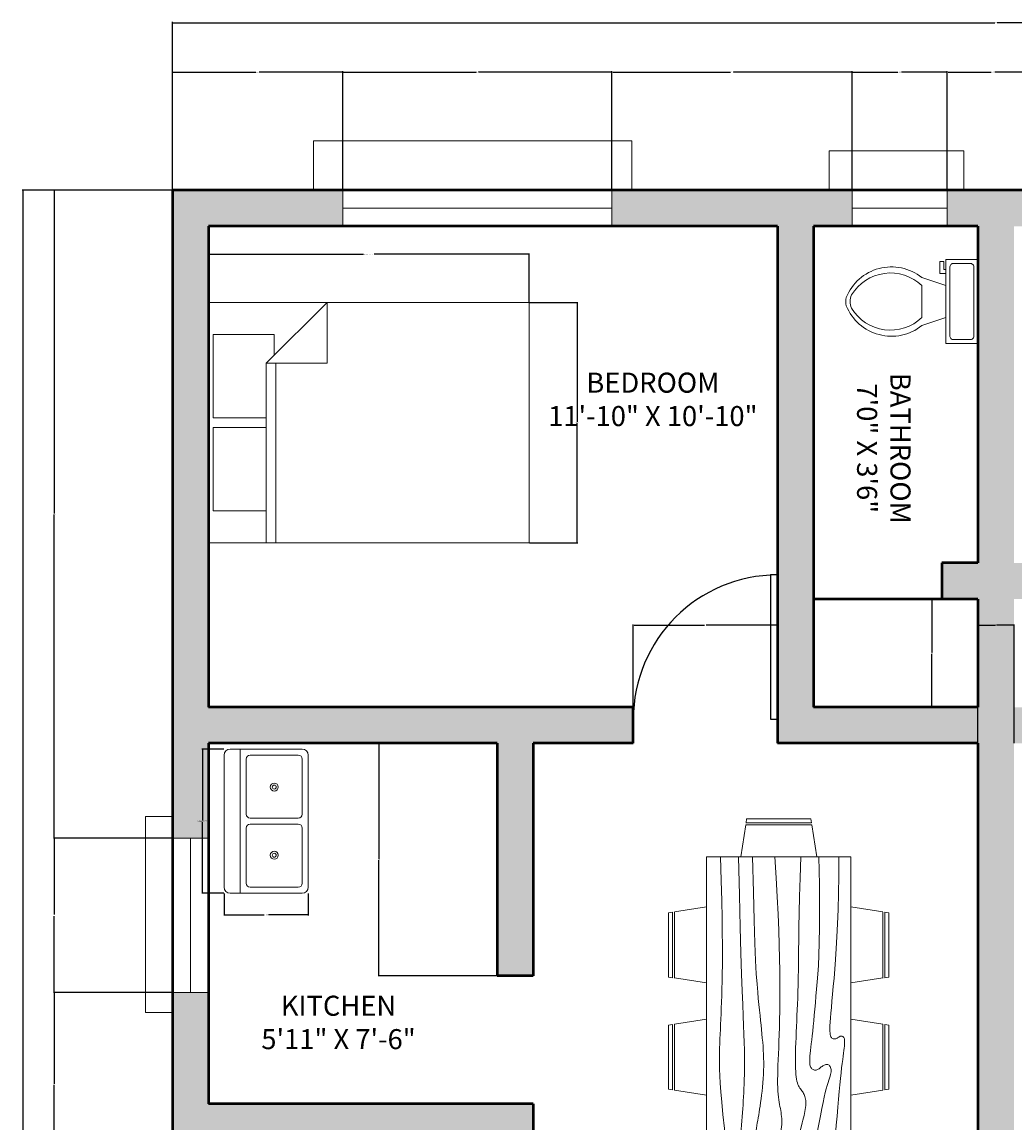
# Model space of a CAD drawing. Units: inches. Extents: x 2710 to 3197, y 524 to 1147.
# Tile 5 of 6: x 2710 to 2957, y 873 to 1147. Entities that reach past the tile are written whole.
import ezdxf

# ---------------------------------------------------------------- set-up
doc = ezdxf.new("R2010")
doc.units = ezdxf.units.IN
for name, color, linetype, lineweight in [('A-ANNO-DIMS', 2, 'Continuous', 18), ('A-AREA-IDEN', 7, 'Continuous', 25), ('A-DOOR', 3, 'Continuous', 25), ('A-FLOR-FIXT', 9, 'Continuous', 20), ('A-FURN', 8, 'Continuous', 18), ('A-GLAZ', 4, 'Continuous', 18), ('A-WALL', 7, 'Continuous', 50), ('A-WALL-PATT', 74, 'Continuous', 13)]:
    doc.layers.add(name, color=color, linetype=linetype, lineweight=lineweight)
doc.styles.get("Standard").update_dxf_attribs({"font": 'arial.ttf'})
doc.dimstyles.get("Standard").update_dxf_attribs({"dimtxt": 0.18, "dimasz": 0.18, "dimexe": 0.18, "dimexo": 0.0625, "dimgap": 0.09, "dimtad": 0, "dimtih": 1, "dimtoh": 1, "dimdec": 4, "dimzin": 0, "dimdsep": 46, "dimtxsty": 'Standard', "dimcen": 0.09, "dimadec": 0, "dimazin": 0, "dimtfac": 1, "dimtdec": 4, "dimtofl": 0, "dimtmove": 0, "dimatfit": 3, "dimfxl": 1, "dimtolj": 1, "dimtzin": 0, "dimarcsym": 0})

# ---------------------------------------------------------------- blocks, each defined once
blk = doc.blocks.new('*U5')
for p, q in [((0, 0), (0, -6)), ((-36, 0), (-36, -6))]:
    blk.add_line(p, q)
blk.add_lwpolyline([(0, 0), (0, 36), (-1.75, 36), (-1.75, 0)], close=True)
blk.add_arc((0, 0), 36, 90, 180)
blk = doc.blocks.new('Toilet - top')
for p, q in [((9.5, -6), (9.5, -2)), ((-8, -8.5), (-8, -8)), ((-7, -8), (-7, -9.5)), ((-4, -8), (-6, -14)), ((4, -8), (6, -14)), ((-10, -8.5), (-8, -8.5)), ((-10, -9.5), (-10, -8.5)), ((-7, -9.5), (-10, -9.5)), ((4, -14), (-4, -14))]:
    blk.add_line(p, q)
blk.add_lwpolyline([(10.5, -8), (10.5, 0), (-10.5, 0), (-10.5, -8)], close=True)
for points in [[(-9.5, -2), (-9.5, -6)], [(8.5, -1), (-8.5, -1)], [(-8.5, -7), (8.5, -7)]]:
    blk.add_lwpolyline(points)
for centre, radius, start, end in [((-8.62, -1.88), 0.884, 81.8699, 188.1301), ((8.62, -1.88), 0.884, 351.8699, 98.1301), ((-8.62, -6.12), 0.884, 171.8699, 278.1301), ((8.62, -6.12), 0.884, 261.8699, 8.1301), ((3.52, -21.58), 12.17, 141.4691, 247.9714), ((4.2, -21.82), 11.33, 136.3677, 238.9468), ((-3.52, -21.58), 12.17, 292.0284, 38.5307), ((-4.2, -21.82), 11.33, 301.053, 43.6321), ((0, -27.88), 4, 245.7318, 294.2682), ((0, -29), 4, 254.8605, 285.1395)]:
    blk.add_arc(centre, radius, start, end)
blk = doc.blocks.new('Bed - Queen')
for p, q in [((0, -80.00003), (0, 0)), ((0, 0), (59.99999, 0)), ((59.99999, 0), (59.99999, -80.00003)), ((7.99999, -1.2), (28.79998, -1.2)), ((7.99999, -14.4), (7.99999, -1.2)), ((28.79998, -1.2), (28.79998, -14.4)), ((31.19999, -1.2), (51.99999, -1.2)), ((31.19999, -14.4), (31.19999, -1.2)), ((51.99999, -1.2), (51.99999, -16.4)), ((0, -14.4), (44.8, -14.4)), ((59.99999, -29.6), (44.8, -14.4)), ((44.8, -14.4), (44.8, -29.6)), ((51.99999, -16.4), (46.79936, -16.4)), ((44.8, -16.8), (0, -16.8)), ((44.8, -29.6), (59.99999, -29.6)), ((59.99999, -80.00003), (0, -80.00003))]:
    blk.add_line(p, q)
blk = doc.blocks.new('Dining Set - 36 x 72 in.')
for p, q in [((-22, 27.5), (-22.1562, 26.50042)), ((-22, 27.5), (-6, 27.5)), ((-5.8437, 26.49966), (-6, 27.5)), ((6, 27.5), (5.8438, 26.50042)), ((6, 27.5), (22, 27.5)), ((22.1563, 26.49966), (22, 27.5)), ((-22.2343, 26.00059), (-23.4847, 17.99762)), ((-22.2304, 26), (-5.7608, 26)), ((-5.8416, 26.5), (-22.1534, 26.5)), ((-4.5152, 17.99762), (-5.7655, 25.99926)), ((5.7657, 26.00059), (4.5153, 17.99762)), ((5.7696, 26), (22.2392, 26)), ((22.1584, 26.5), (5.8466, 26.5)), ((23.4848, 17.99762), (22.2345, 25.99926)), ((36, 18), (-36, 18)), ((-36, 18), (-36, -18)), ((36, -18), (36, 18)), ((-44.0006, 8.23428), (-35.9976, 9.48474)), ((44.0006, 8.23428), (35.9976, 9.48474)), ((-45.5, 8), (-44.5004, 8.15617)), ((-45.5, 8), (-45.5, -8)), ((-44.5, -8.15843), (-44.5, 8.15338)), ((-44, 8.23041), (-44, -8.23915)), ((44, 8.23041), (44, -8.23915)), ((44.5, -8.15843), (44.5, 8.15338)), ((45.5, 8), (44.5005, 8.15617)), ((45.5, 8), (45.5, -8)), ((-44.4997, -8.15631), (-45.5, -8)), ((-35.9976, -9.48476), (-43.9993, -8.2345)), ((35.9976, -9.48476), (43.9993, -8.2345)), ((44.4997, -8.15631), (45.5, -8)), ((-36, -18), (36, -18)), ((-22.2343, -26.0006), (-23.4847, -17.99762)), ((-4.5152, -17.99762), (-5.7655, -25.99928)), ((5.7657, -26.0006), (4.5153, -17.99762)), ((23.4848, -17.99762), (22.2345, -25.99928)), ((-22.2304, -26), (-5.7608, -26)), ((-22, -27.5), (-22.1562, -26.50044)), ((-5.8416, -26.5), (-22.1534, -26.5)), ((-5.8437, -26.49967), (-6, -27.5)), ((5.7696, -26), (22.2392, -26)), ((6, -27.5), (5.8438, -26.50044)), ((22.1584, -26.5), (5.8466, -26.5)), ((22.1563, -26.49967), (22, -27.5)), ((-22, -27.5), (-6, -27.5)), ((6, -27.5), (22, -27.5))]:
    blk.add_line(p, q)
for points in [[(-36, 15), (-31.1772, 14.97754), (-26.8079, 14.91406), (-22.8538, 14.81543), (-19.276, 14.6875), (-16.0362, 14.53613), (-13.0957, 14.36718), (-10.4159, 14.18652), (-7.9583, 14), (-5.6904, 13.81315), (-3.6035, 13.63021), (-1.6954, 13.45508), (0.0365, 13.29166), (1.5945, 13.14388), (2.9811, 13.01562), (4.1988, 12.9108), (5.25, 12.83333), (6.1393, 12.78613), (6.8802, 12.76823), (7.4883, 12.77767), (7.9792, 12.8125), (8.3685, 12.87077), (8.6719, 12.95052), (8.9049, 13.0498), (9.0833, 13.16666), (9.2205, 13.29899), (9.3216, 13.44401), (9.3895, 13.59879), (9.4271, 13.76041), (9.4373, 13.92594), (9.4232, 14.09245), (9.3875, 14.257), (9.3333, 14.41666), (9.2638, 14.56917), (9.1836, 14.71484), (9.0975, 14.85465), (9.0104, 14.98958), (8.9272, 15.1206), (8.8529, 15.2487), (8.7922, 15.37483), (8.75, 15.5), (8.7305, 15.62467), (8.7344, 15.74739), (8.7617, 15.86621), (8.8125, 15.97916), (8.8867, 16.08431), (8.9844, 16.17968), (9.1055, 16.26334), (9.25, 16.33333), (9.4189, 16.38802), (9.6172, 16.42708), (9.8506, 16.45052), (10.125, 16.45833), (10.4463, 16.45052), (10.8203, 16.42708), (11.2529, 16.38802), (11.75, 16.33333), (12.3184, 16.26318), (12.9694, 16.17838), (13.7151, 16.07991), (14.5677, 15.96875), (15.5395, 15.84586), (16.6426, 15.71224), (17.8893, 15.56884), (19.2917, 15.41666), (20.859, 15.25667), (22.5879, 15.08984), (24.4721, 14.91715), (26.5052, 14.73958), (28.6809, 14.5581), (30.9929, 14.3737), (33.4347, 14.18733), (36, 14)], [(-36, 10), (-28.9766, 10.14274), (-23.1725, 10.20442), (-18.4241, 10.19775), (-14.5677, 10.13541), (-11.4399, 10.03011), (-8.877, 9.89453), (-6.7154, 9.74137), (-4.7917, 9.58333), (-2.9698, 9.43082), (-1.2246, 9.28515), (0.4415, 9.14534), (2.026, 9.01041), (3.5266, 8.87939), (4.9408, 8.7513), (6.266, 8.62516), (7.5, 8.5), (8.6411, 8.37549), (9.6914, 8.2539), (10.6538, 8.13818), (11.5312, 8.03125), (12.3267, 7.93603), (13.043, 7.85547), (13.6831, 7.79248), (14.25, 7.75), (14.7471, 7.7303), (15.1797, 7.73307), (15.5537, 7.75732), (15.875, 7.80208), (16.1494, 7.86637), (16.3828, 7.94922), (16.5811, 8.04964), (16.75, 8.16666), (16.8944, 8.29915), (17.0143, 8.44531), (17.1089, 8.60319), (17.1771, 8.77083), (17.218, 8.94629), (17.2305, 9.1276), (17.2137, 9.31282), (17.1667, 9.5), (17.0895, 9.6875), (16.987, 9.875), (16.8649, 10.0625), (16.7292, 10.25), (16.5856, 10.4375), (16.4401, 10.625), (16.2985, 10.8125), (16.1667, 11), (16.05, 11.18733), (15.9518, 11.3737), (15.8752, 11.5581), (15.8229, 11.73958), (15.798, 11.91715), (15.8034, 12.08984), (15.842, 12.25667), (15.9167, 12.41666), (16.0295, 12.56836), (16.1784, 12.70833), (16.3605, 12.83268), (16.5729, 12.9375), (16.8127, 13.01888), (17.0768, 13.07291), (17.3625, 13.0957), (17.6667, 13.08333), (17.9894, 13.03312), (18.3418, 12.94726), (18.7382, 12.82918), (19.1927, 12.68229), (19.7195, 12.51001), (20.3327, 12.31575), (21.0465, 12.10294), (21.875, 11.875), (22.8357, 11.63354), (23.959, 11.37304), (25.2786, 11.08618), (26.8282, 10.76562), (28.6414, 10.40405), (30.752, 9.99414), (33.1936, 9.52856), (36, 9)], [(-36, 5.5), (-30.7157, 5.3348), (-26.069, 5.20963), (-21.9946, 5.11767), (-18.4271, 5.05208), (-15.3009, 5.00602), (-12.5508, 4.97265), (-10.1112, 4.94515), (-7.9167, 4.91666), (-5.909, 4.88167), (-4.0586, 4.83984), (-2.3429, 4.79215), (-0.7396, 4.73958), (0.7739, 4.6831), (2.22, 4.6237), (3.6213, 4.56233), (5, 4.5), (6.373, 4.43782), (7.7344, 4.3776), (9.0723, 4.32129), (10.375, 4.27083), (11.6309, 4.22819), (12.8281, 4.19531), (13.9551, 4.17415), (15, 4.16666), (15.954, 4.17448), (16.819, 4.19791), (17.6001, 4.23698), (18.3021, 4.29166), (18.9299, 4.36198), (19.4883, 4.44791), (19.9823, 4.54948), (20.4167, 4.66666), (20.7969, 4.79899), (21.1302, 4.94401), (21.4245, 5.09879), (21.6875, 5.26041), (21.9271, 5.42594), (22.1511, 5.59245), (22.3672, 5.757), (22.5834, 5.91666), (22.8065, 6.06868), (23.0404, 6.21093), (23.2879, 6.34147), (23.5521, 6.45833), (23.8358, 6.55957), (24.142, 6.64323), (24.4735, 6.70735), (24.8334, 6.75), (25.2235, 6.76969), (25.642, 6.76692), (26.0858, 6.74267), (26.5521, 6.69791), (27.0379, 6.63362), (27.5404, 6.55078), (28.0565, 6.45036), (28.5834, 6.33333), (29.1242, 6.19987), (29.7071, 6.04687), (30.3661, 5.87044), (31.1354, 5.66666), (32.0493, 5.43164), (33.142, 5.16146), (34.4475, 4.85221), (36, 4.5)], [(-36, -1), (-30.7915, -0.6591), (-26.0195, -0.38216), (-21.6519, -0.16284), (-17.6563, 0.00521), (-14.0005, 0.12833), (-10.6523, 0.21289), (-7.5796, 0.26522), (-4.75, 0.29166), (-2.134, 0.29793), (0.2878, 0.28711), (2.5317, 0.26163), (4.6146, 0.22396), (6.5529, 0.17651), (8.3633, 0.12174), (10.0623, 0.06209), (11.6667, 0), (13.1899, -0.06201), (14.6341, -0.1211), (15.9982, -0.17432), (17.2813, -0.21875), (18.4823, -0.25147), (19.6003, -0.26953), (20.6343, -0.27002), (21.5834, -0.25), (22.4481, -0.20768), (23.2357, -0.14584), (23.9549, -0.06836), (24.6146, 0.02083), (25.2235, 0.11784), (25.7904, 0.21875), (26.3241, 0.31966), (26.8334, 0.41666), (27.3265, 0.50618), (27.8099, 0.58593), (28.2894, 0.65397), (28.7709, 0.70833), (29.2601, 0.74707), (29.763, 0.76823), (30.2855, 0.76985), (30.8334, 0.75), (31.4088, 0.70784), (31.9994, 0.64713), (32.589, 0.57275), (33.1615, 0.48958), (33.7008, 0.4025), (34.1908, 0.3164), (34.6153, 0.23616), (34.9584, 0.16666), (35.2099, 0.11165), (35.3848, 0.07031), (35.504, 0.04069), (35.5886, 0.02083), (35.6594, 0.00879), (35.7377, 0.0026), (35.8442, 0.00032), (36, 0)], [(-36, -6.5), (-27.1843, -6.31267), (-20.084, -6.1263), (-14.469, -5.9419), (-10.1094, -5.76042), (-6.7752, -5.58285), (-4.2363, -5.41016), (-2.2629, -5.24333), (-0.625, -5.08334), (0.8708, -4.93099), (2.2715, -4.78646), (3.5872, -4.64974), (4.8281, -4.52084), (6.0046, -4.39974), (7.127, -4.28646), (8.2053, -4.18099), (9.25, -4.08334), (10.2705, -3.99382), (11.2734, -3.91407), (12.2647, -3.84603), (13.25, -3.79167), (14.2354, -3.75293), (15.2266, -3.73177), (16.2295, -3.73015), (17.25, -3.75), (18.2912, -3.79248), (19.3451, -3.85547), (20.4009, -3.93604), (21.4479, -4.03125), (22.4754, -4.13819), (23.4727, -4.25391), (24.4289, -4.37549), (25.3334, -4.5), (26.1785, -4.62492), (26.9694, -4.74935), (27.7145, -4.87281), (28.4219, -4.99479), (29.1, -5.11483), (29.7572, -5.23242), (30.4016, -5.34709), (31.0417, -5.45834), (31.6837, -5.56437), (32.3262, -5.65821), (32.9658, -5.73153), (33.599, -5.77604), (34.2224, -5.78345), (34.8327, -5.74545), (35.4264, -5.65373), (36, -5.5)], [(-36, -10), (-26.4022, -9.81299), (-18.4675, -9.62891), (-11.9839, -9.45069), (-6.7396, -9.28125), (-2.5226, -9.12354), (0.8789, -8.98047), (3.6769, -8.85498), (6.0833, -8.75), (8.2767, -8.66765), (10.3021, -8.60677), (12.1712, -8.56543), (13.8958, -8.54167), (15.4876, -8.53353), (16.9583, -8.53907), (18.3197, -8.55632), (19.5834, -8.58334), (20.7616, -8.61841), (21.8685, -8.66081), (22.9188, -8.71004), (23.9271, -8.76563), (24.9081, -8.82707), (25.8763, -8.89388), (26.8465, -8.96558), (27.8334, -9.04167), (28.8474, -9.12118), (29.8828, -9.20117), (30.93, -9.27824), (31.9792, -9.34896), (33.0205, -9.40991), (34.0443, -9.45768), (35.0407, -9.48885), (36, -9.5)], [(-36, -14.5), (-30.0881, -14.33513), (-25.0332, -14.21224), (-20.7312, -14.12647), (-17.0781, -14.07292), (-13.97, -14.04671), (-11.3027, -14.04297), (-8.9724, -14.05681), (-6.875, -14.08334), (-4.9224, -14.11833), (-3.0905, -14.16016), (-1.3709, -14.20785), (0.2448, -14.26042), (1.7647, -14.3169), (3.1973, -14.3763), (4.5507, -14.43767), (5.8333, -14.5), (7.0554, -14.5621), (8.235, -14.62175), (9.3922, -14.67652), (10.5469, -14.72396), (11.7192, -14.76164), (12.929, -14.78711), (14.1965, -14.79794), (15.5417, -14.79167), (16.9933, -14.76424), (18.6152, -14.70508), (20.4804, -14.60197), (22.6615, -14.44271), (25.2312, -14.21509), (28.2624, -13.9069), (31.8277, -13.50594), (36, -13)]]:
    blk.add_lwpolyline(points)
blk = doc.blocks.new('Sink-double - 36 in top')
for p, q in [((-18, -4), (18, -4)), ((-0.75, -18.5), (-0.75, -6.5)), ((0.75, -6.5), (0.75, -18.5))]:
    blk.add_line(p, q)
for points in [[(-16.5, 0), (16.5, 0)], [(-18, -19.5), (-18, -1.5)], [(18, -1.5), (18, -19.5)], [(-16.5, -18.5), (-16.5, -6.5)], [(-15.5, -5.5), (-1.75, -5.5)], [(1.75, -5.5), (15.5, -5.5)], [(16.5, -6.5), (16.5, -18.5)], [(16.5, -21), (-16.5, -21)], [(-1.75, -19.5), (-15.5, -19.5)], [(15.5, -19.5), (1.75, -19.5)]]:
    blk.add_lwpolyline(points)
for centre, radius in [((-8.5, -12.5), 1), ((-8.5, -12.5), 0.5), ((8.5, -12.5), 1), ((8.5, -12.5), 0.5)]:
    blk.add_circle(centre, radius)
for centre, radius, start, end in [((-16.5, -1.5), 1.5, 90, 180), ((16.5, -1.5), 1.5, 0, 90), ((-15.5, -6.5), 1, 90, 180), ((-1.75, -6.5), 1, 0, 90), ((1.75, -6.5), 1, 90, 180), ((15.5, -6.5), 1, 0, 90), ((-15.5, -18.5), 1, 180, 270), ((-1.75, -18.5), 1, 270, 0), ((1.75, -18.5), 1, 180, 270), ((15.5, -18.5), 1, 270, 0), ((-16.5, -19.5), 1.5, 180, 270), ((16.5, -19.5), 1.5, 270, 0)]:
    blk.add_arc(centre, radius, start, end)
blk = doc.blocks.new('*D22')
at = {"layer": 'A-ANNO-DIMS', "color": 0, "lineweight": -2, "transparency": 16777216}
for p, q in [((2756.35, 1077.1), (2756.35, 1089.21)), ((2756.53, 1089.03), (2795.05, 1089.03)), ((2836.17, 1089.03), (2797.65, 1089.03)), ((2836.35, 1077.1), (2836.35, 1089.21))]:
    blk.add_line(p, q, dxfattribs=at)
at = {"layer": 'A-ANNO-DIMS', "color": 0, "transparency": 16777216}
for points in [[(2756.53, 1089.06), (2756.53, 1089), (2756.35, 1089.03)], [(2836.17, 1089.06), (2836.17, 1089), (2836.35, 1089.03)]]:
    blk.add_solid(points, dxfattribs=at)
at = {"layer": 'Defpoints', "color": 0, "transparency": 16777216}
for p in [(2756.35, 1089.03), (2756.35, 1077.03), (2836.35, 1077.03)]:
    blk.add_point(p, dxfattribs=at)
at = {"layer": 'A-ANNO-DIMS', "color": 0, "transparency": 16777216, "insert": (2796.35, 1089.03), "char_height": 0.18, "attachment_point": 5}
blk.add_mtext('\\A1;QUEEN BED 80 TYP.', dxfattribs=at)
blk = doc.blocks.new('*D23')
at = {"layer": 'A-ANNO-DIMS', "color": 0, "lineweight": -2, "transparency": 16777216}
for p, q in [((2836.41, 1077.03), (2848.53, 1077.03)), ((2848.35, 1076.85), (2848.35, 1047.22)), ((2848.35, 1017.21), (2848.35, 1046.85)), ((2836.41, 1017.03), (2848.53, 1017.03))]:
    blk.add_line(p, q, dxfattribs=at)
at = {"layer": 'A-ANNO-DIMS', "color": 0, "transparency": 16777216}
for points in [[(2848.32, 1076.85), (2848.38, 1076.85), (2848.35, 1077.03)], [(2848.32, 1017.21), (2848.38, 1017.21), (2848.35, 1017.03)]]:
    blk.add_solid(points, dxfattribs=at)
at = {"layer": 'Defpoints', "color": 0, "transparency": 16777216}
for p in [(2836.35, 1077.03), (2848.35, 1077.03), (2836.35, 1017.03)]:
    blk.add_point(p, dxfattribs=at)
at = {"layer": 'A-ANNO-DIMS', "color": 0, "transparency": 16777216, "insert": (2848.35, 1047.03), "char_height": 0.18, "attachment_point": 5}
blk.add_mtext('\\A1;60 TYP.', dxfattribs=at)
blk = doc.blocks.new('*D28')
at = {"layer": 'A-ANNO-DIMS', "color": 0, "lineweight": -2, "transparency": 16777216}
for p, q in [((2760.19, 965.57), (2754.67, 965.57)), ((2754.85, 965.39), (2754.85, 947.76)), ((2754.85, 929.75), (2754.85, 947.39)), ((2760.19, 929.57), (2754.67, 929.57))]:
    blk.add_line(p, q, dxfattribs=at)
at = {"layer": 'A-ANNO-DIMS', "color": 0, "transparency": 16777216}
for points in [[(2754.82, 965.39), (2754.88, 965.39), (2754.85, 965.57)], [(2754.82, 929.75), (2754.88, 929.75), (2754.85, 929.57)]]:
    blk.add_solid(points, dxfattribs=at)
at = {"layer": 'Defpoints', "color": 0, "transparency": 16777216}
for p in [(2754.85, 965.57), (2760.25, 965.57), (2760.25, 929.57)]:
    blk.add_point(p, dxfattribs=at)
at = {"layer": 'A-ANNO-DIMS', "color": 0, "transparency": 16777216, "insert": (2754.85, 947.57), "char_height": 0.18, "attachment_point": 5}
blk.add_mtext('\\A1;DOUBLE SINK 36 TYP.', dxfattribs=at)
blk = doc.blocks.new('*D29')
at = {"layer": 'A-ANNO-DIMS', "color": 0, "lineweight": -2, "transparency": 16777216}
for p, q in [((2760.25, 929.51), (2760.25, 923.99)), ((2781.25, 929.51), (2781.25, 923.99)), ((2760.43, 924.17), (2770.22, 924.17)), ((2781.07, 924.17), (2771.28, 924.17))]:
    blk.add_line(p, q, dxfattribs=at)
at = {"layer": 'A-ANNO-DIMS', "color": 0, "transparency": 16777216}
for points in [[(2760.43, 924.2), (2760.43, 924.14), (2760.25, 924.17)], [(2781.07, 924.2), (2781.07, 924.14), (2781.25, 924.17)]]:
    blk.add_solid(points, dxfattribs=at)
at = {"layer": 'Defpoints', "color": 0, "transparency": 16777216}
for p in [(2760.25, 929.57), (2781.25, 929.57), (2760.25, 924.17)]:
    blk.add_point(p, dxfattribs=at)
at = {"layer": 'A-ANNO-DIMS', "color": 0, "transparency": 16777216, "insert": (2770.75, 924.17), "char_height": 0.18, "attachment_point": 5}
blk.add_mtext('\\A1;21 TYP.', dxfattribs=at)
blk = doc.blocks.new('*D34')
at = {"layer": 'A-ANNO-DIMS', "color": 0, "lineweight": -2, "transparency": 16777216}
for p, q in [((2747.35, 1105.06), (2747.35, 1146.99)), ((2747.53, 1146.81), (2952.57, 1146.81)), ((3158.17, 1146.81), (2953.12, 1146.81)), ((3158.35, 1105.06), (3158.35, 1146.99))]:
    blk.add_line(p, q, dxfattribs=at)
at = {"layer": 'A-ANNO-DIMS', "color": 0, "transparency": 16777216}
for points in [[(2747.53, 1146.84), (2747.53, 1146.78), (2747.35, 1146.81)], [(3158.17, 1146.84), (3158.17, 1146.78), (3158.35, 1146.81)]]:
    blk.add_solid(points, dxfattribs=at)
at = {"layer": 'Defpoints', "color": 0, "transparency": 16777216}
for p in [(3158.35, 1146.81), (2747.35, 1105), (3158.35, 1105)]:
    blk.add_point(p, dxfattribs=at)
at = {"layer": 'A-ANNO-DIMS', "color": 0, "transparency": 16777216, "insert": (2952.85, 1146.81), "char_height": 0.18, "attachment_point": 5}
blk.add_mtext('\\A1;411', dxfattribs=at)
blk = doc.blocks.new('*D35')
at = {"layer": 'A-ANNO-DIMS', "color": 0, "lineweight": -2, "transparency": 16777216}
for p, q in [((2747.29, 1105), (2709.83, 1105)), ((2710.01, 1104.82), (2710.01, 835.18)), ((2710.01, 565.18), (2710.01, 834.82)), ((2747.29, 565), (2709.83, 565))]:
    blk.add_line(p, q, dxfattribs=at)
at = {"layer": 'A-ANNO-DIMS', "color": 0, "transparency": 16777216}
for points in [[(2709.98, 1104.82), (2710.04, 1104.82), (2710.01, 1105)], [(2709.98, 565.18), (2710.04, 565.18), (2710.01, 565)]]:
    blk.add_solid(points, dxfattribs=at)
at = {"layer": 'Defpoints', "color": 0, "transparency": 16777216}
for p in [(2710.01, 1105), (2747.35, 1105), (2747.35, 565)]:
    blk.add_point(p, dxfattribs=at)
at = {"layer": 'A-ANNO-DIMS', "color": 0, "transparency": 16777216, "insert": (2710.01, 835), "char_height": 0.18, "attachment_point": 5}
blk.add_mtext('\\A1;540', dxfattribs=at)
blk = doc.blocks.new('*D36')
at = {"layer": 'A-ANNO-DIMS', "color": 0, "lineweight": -2, "transparency": 16777216}
for p, q in [((2747.35, 1105.06), (2747.35, 1134.68)), ((2747.53, 1134.5), (2768.19, 1134.5)), ((2789.65, 1134.5), (2768.99, 1134.5)), ((2789.83, 1105.06), (2789.83, 1134.68))]:
    blk.add_line(p, q, dxfattribs=at)
at = {"layer": 'A-ANNO-DIMS', "color": 0, "transparency": 16777216}
for points in [[(2747.53, 1134.53), (2747.53, 1134.47), (2747.35, 1134.5)], [(2789.65, 1134.53), (2789.65, 1134.47), (2789.83, 1134.5)]]:
    blk.add_solid(points, dxfattribs=at)
at = {"layer": 'Defpoints', "color": 0, "transparency": 16777216}
for p in [(2789.83, 1134.5), (2747.35, 1105), (2789.83, 1105)]:
    blk.add_point(p, dxfattribs=at)
at = {"layer": 'A-ANNO-DIMS', "color": 0, "transparency": 16777216, "insert": (2768.59, 1134.5), "char_height": 0.18, "attachment_point": 5}
blk.add_mtext('\\A1;42.48', dxfattribs=at)
blk = doc.blocks.new('*D37')
at = {"layer": 'A-ANNO-DIMS', "color": 0, "lineweight": -2, "transparency": 16777216}
for p, q in [((2789.83, 1105.06), (2789.83, 1134.68)), ((2790.01, 1134.5), (2823.11, 1134.5)), ((2856.85, 1134.5), (2823.75, 1134.5)), ((2857.03, 1105.06), (2857.03, 1134.68))]:
    blk.add_line(p, q, dxfattribs=at)
at = {"layer": 'A-ANNO-DIMS', "color": 0, "transparency": 16777216}
for points in [[(2790.01, 1134.53), (2790.01, 1134.47), (2789.83, 1134.5)], [(2856.85, 1134.53), (2856.85, 1134.47), (2857.03, 1134.5)]]:
    blk.add_solid(points, dxfattribs=at)
at = {"layer": 'Defpoints', "color": 0, "transparency": 16777216}
for p in [(2857.03, 1134.5), (2789.83, 1105), (2857.03, 1105)]:
    blk.add_point(p, dxfattribs=at)
at = {"layer": 'A-ANNO-DIMS', "color": 0, "transparency": 16777216, "insert": (2823.43, 1134.5), "char_height": 0.18, "attachment_point": 5}
blk.add_mtext('\\A1;67.2', dxfattribs=at)
blk = doc.blocks.new('*D38')
at = {"layer": 'A-ANNO-DIMS', "color": 0, "lineweight": -2, "transparency": 16777216}
for p, q in [((2857.03, 1105.06), (2857.03, 1134.68)), ((2857.21, 1134.5), (2886.6, 1134.5)), ((2916.78, 1134.5), (2887.39, 1134.5)), ((2916.96, 1105.06), (2916.96, 1134.68))]:
    blk.add_line(p, q, dxfattribs=at)
at = {"layer": 'A-ANNO-DIMS', "color": 0, "transparency": 16777216}
for points in [[(2857.21, 1134.53), (2857.21, 1134.47), (2857.03, 1134.5)], [(2916.78, 1134.53), (2916.78, 1134.47), (2916.96, 1134.5)]]:
    blk.add_solid(points, dxfattribs=at)
at = {"layer": 'Defpoints', "color": 0, "transparency": 16777216}
for p in [(2916.96, 1134.5), (2857.03, 1105), (2916.96, 1105)]:
    blk.add_point(p, dxfattribs=at)
at = {"layer": 'A-ANNO-DIMS', "color": 0, "transparency": 16777216, "insert": (2886.99, 1134.5), "char_height": 0.18, "attachment_point": 5}
blk.add_mtext('\\A1;59.93', dxfattribs=at)
blk = doc.blocks.new('*D39')
at = {"layer": 'A-ANNO-DIMS', "color": 0, "lineweight": -2, "transparency": 16777216}
for p, q in [((2916.96, 1105.06), (2916.96, 1134.68)), ((2917.14, 1134.5), (2928.37, 1134.5)), ((2940.52, 1134.5), (2929.3, 1134.5)), ((2940.7, 1105.06), (2940.7, 1134.68))]:
    blk.add_line(p, q, dxfattribs=at)
at = {"layer": 'A-ANNO-DIMS', "color": 0, "transparency": 16777216}
for points in [[(2917.14, 1134.53), (2917.14, 1134.47), (2916.96, 1134.5)], [(2940.52, 1134.53), (2940.52, 1134.47), (2940.7, 1134.5)]]:
    blk.add_solid(points, dxfattribs=at)
at = {"layer": 'Defpoints', "color": 0, "transparency": 16777216}
for p in [(2940.7, 1134.5), (2916.96, 1105), (2940.7, 1105)]:
    blk.add_point(p, dxfattribs=at)
at = {"layer": 'A-ANNO-DIMS', "color": 0, "transparency": 16777216, "insert": (2928.83, 1134.5), "char_height": 0.18, "attachment_point": 5}
blk.add_mtext('\\A1;23.743', dxfattribs=at)
blk = doc.blocks.new('*D40')
at = {"layer": 'A-ANNO-DIMS', "color": 0, "lineweight": -2, "transparency": 16777216}
for p, q in [((2940.7, 1105.06), (2940.7, 1134.68)), ((2940.88, 1134.5), (2951.61, 1134.5)), ((2963.27, 1134.5), (2952.54, 1134.5)), ((2963.45, 1105.06), (2963.45, 1134.68))]:
    blk.add_line(p, q, dxfattribs=at)
at = {"layer": 'A-ANNO-DIMS', "color": 0, "transparency": 16777216}
for points in [[(2940.88, 1134.53), (2940.88, 1134.47), (2940.7, 1134.5)], [(2963.27, 1134.53), (2963.27, 1134.47), (2963.45, 1134.5)]]:
    blk.add_solid(points, dxfattribs=at)
at = {"layer": 'Defpoints', "color": 0, "transparency": 16777216}
for p in [(2963.45, 1134.5), (2940.7, 1105), (2963.45, 1105)]:
    blk.add_point(p, dxfattribs=at)
at = {"layer": 'A-ANNO-DIMS', "color": 0, "transparency": 16777216, "insert": (2952.08, 1134.5), "char_height": 0.18, "attachment_point": 5}
blk.add_mtext('\\A1;22.746', dxfattribs=at)
blk = doc.blocks.new('*D54')
at = {"layer": 'A-ANNO-DIMS', "color": 0, "lineweight": -2, "transparency": 16777216}
for p, q in [((2747.29, 904.83), (2717.67, 904.83)), ((2717.85, 904.65), (2717.85, 882.03)), ((2717.85, 859.04), (2717.85, 881.66)), ((2747.29, 858.86), (2717.67, 858.86))]:
    blk.add_line(p, q, dxfattribs=at)
at = {"layer": 'A-ANNO-DIMS', "color": 0, "transparency": 16777216}
for points in [[(2717.82, 904.65), (2717.88, 904.65), (2717.85, 904.83)], [(2717.82, 859.04), (2717.88, 859.04), (2717.85, 858.86)]]:
    blk.add_solid(points, dxfattribs=at)
at = {"layer": 'Defpoints', "color": 0, "transparency": 16777216}
for p in [(2717.85, 904.83), (2747.35, 904.83), (2747.35, 858.86)]:
    blk.add_point(p, dxfattribs=at)
at = {"layer": 'A-ANNO-DIMS', "color": 0, "transparency": 16777216, "insert": (2717.85, 881.84), "char_height": 0.18, "attachment_point": 5}
blk.add_mtext('\\A1;45.98', dxfattribs=at)
blk = doc.blocks.new('*D55')
at = {"layer": 'A-ANNO-DIMS', "color": 0, "lineweight": -2, "transparency": 16777216}
for p, q in [((2747.29, 943.33), (2717.67, 943.33)), ((2717.85, 943.15), (2717.85, 924.26)), ((2717.85, 905.01), (2717.85, 923.9)), ((2747.29, 904.83), (2717.67, 904.83))]:
    blk.add_line(p, q, dxfattribs=at)
at = {"layer": 'A-ANNO-DIMS', "color": 0, "transparency": 16777216}
for points in [[(2717.82, 943.15), (2717.88, 943.15), (2717.85, 943.33)], [(2717.82, 905.01), (2717.88, 905.01), (2717.85, 904.83)]]:
    blk.add_solid(points, dxfattribs=at)
at = {"layer": 'Defpoints', "color": 0, "transparency": 16777216}
for p in [(2717.85, 943.33), (2747.35, 943.33), (2747.35, 904.83)]:
    blk.add_point(p, dxfattribs=at)
at = {"layer": 'A-ANNO-DIMS', "color": 0, "transparency": 16777216, "insert": (2717.85, 924.08), "char_height": 0.18, "attachment_point": 5}
blk.add_mtext('\\A1;38.49', dxfattribs=at)
blk = doc.blocks.new('*D56')
at = {"layer": 'A-ANNO-DIMS', "color": 0, "lineweight": -2, "transparency": 16777216}
for p, q in [((2747.29, 1105), (2717.67, 1105)), ((2717.85, 1104.82), (2717.85, 1024.35)), ((2717.85, 943.51), (2717.85, 1023.98)), ((2747.29, 943.33), (2717.67, 943.33))]:
    blk.add_line(p, q, dxfattribs=at)
at = {"layer": 'A-ANNO-DIMS', "color": 0, "transparency": 16777216}
for points in [[(2717.82, 1104.82), (2717.88, 1104.82), (2717.85, 1105)], [(2717.82, 943.51), (2717.88, 943.51), (2717.85, 943.33)]]:
    blk.add_solid(points, dxfattribs=at)
at = {"layer": 'Defpoints', "color": 0, "transparency": 16777216}
for p in [(2717.85, 1105), (2747.35, 1105), (2747.35, 943.33)]:
    blk.add_point(p, dxfattribs=at)
at = {"layer": 'A-ANNO-DIMS', "color": 0, "transparency": 16777216, "insert": (2717.85, 1024.16), "char_height": 0.18, "attachment_point": 5}
blk.add_mtext('\\A1;161.67', dxfattribs=at)
blk = doc.blocks.new('*D74')
at = {"layer": 'A-ANNO-DIMS', "color": 0, "lineweight": -2, "transparency": 16777216}
for p, q in [((2862.35, 967.06), (2862.35, 996.68)), ((2862.53, 996.5), (2880.13, 996.5)), ((2898.17, 996.5), (2880.57, 996.5)), ((2898.35, 967.06), (2898.35, 996.68))]:
    blk.add_line(p, q, dxfattribs=at)
at = {"layer": 'A-ANNO-DIMS', "color": 0, "transparency": 16777216}
for points in [[(2862.53, 996.53), (2862.53, 996.47), (2862.35, 996.5)], [(2898.17, 996.53), (2898.17, 996.47), (2898.35, 996.5)]]:
    blk.add_solid(points, dxfattribs=at)
at = {"layer": 'Defpoints', "color": 0, "transparency": 16777216}
for p in [(2898.35, 996.5), (2862.35, 967), (2898.35, 967)]:
    blk.add_point(p, dxfattribs=at)
at = {"layer": 'A-ANNO-DIMS', "color": 0, "transparency": 16777216, "insert": (2880.35, 996.5), "char_height": 0.18, "attachment_point": 5}
blk.add_mtext('\\A1;36', dxfattribs=at)
blk = doc.blocks.new('*D77')
at = {"layer": 'A-ANNO-DIMS', "color": 0, "lineweight": -2, "transparency": 16777216}
for p, q in [((2948.35, 967.06), (2948.35, 996.68)), ((2948.53, 996.5), (2952.7, 996.5)), ((2957.17, 996.5), (2953, 996.5)), ((2957.35, 967.06), (2957.35, 996.68))]:
    blk.add_line(p, q, dxfattribs=at)
at = {"layer": 'A-ANNO-DIMS', "color": 0, "transparency": 16777216}
for points in [[(2948.53, 996.53), (2948.53, 996.47), (2948.35, 996.5)], [(2957.17, 996.53), (2957.17, 996.47), (2957.35, 996.5)]]:
    blk.add_solid(points, dxfattribs=at)
at = {"layer": 'Defpoints', "color": 0, "transparency": 16777216}
for p in [(2957.35, 996.5), (2948.35, 967), (2957.35, 967)]:
    blk.add_point(p, dxfattribs=at)
at = {"layer": 'A-ANNO-DIMS', "color": 0, "transparency": 16777216, "insert": (2952.85, 996.5), "char_height": 0.18, "attachment_point": 5}
blk.add_mtext('\\A1;9', dxfattribs=at)
blk = doc.blocks.new('*D82')
at = {"layer": 'A-ANNO-DIMS', "color": 0, "lineweight": -2, "transparency": 16777216}
for p, q in [((2907.41, 1003), (2937.03, 1003)), ((2936.85, 1002.82), (2936.85, 989.68)), ((2936.85, 976.18), (2936.85, 989.32)), ((2907.41, 976), (2937.03, 976))]:
    blk.add_line(p, q, dxfattribs=at)
at = {"layer": 'A-ANNO-DIMS', "color": 0, "transparency": 16777216}
for points in [[(2936.82, 1002.82), (2936.88, 1002.82), (2936.85, 1003)], [(2936.82, 976.18), (2936.88, 976.18), (2936.85, 976)]]:
    blk.add_solid(points, dxfattribs=at)
at = {"layer": 'Defpoints', "color": 0, "transparency": 16777216}
for p in [(2907.35, 1003), (2907.35, 976), (2936.85, 976)]:
    blk.add_point(p, dxfattribs=at)
at = {"layer": 'A-ANNO-DIMS', "color": 0, "transparency": 16777216, "insert": (2936.85, 989.5), "char_height": 0.18, "attachment_point": 5}
blk.add_mtext('\\A1;27', dxfattribs=at)
blk = doc.blocks.new('*D83')
at = {"layer": 'A-ANNO-DIMS', "color": 0, "lineweight": -2, "transparency": 16777216}
for p, q in [((2828.29, 967), (2798.67, 967)), ((2798.85, 966.82), (2798.85, 938.18)), ((2798.85, 909.18), (2798.85, 937.82)), ((2828.29, 909), (2798.67, 909))]:
    blk.add_line(p, q, dxfattribs=at)
at = {"layer": 'A-ANNO-DIMS', "color": 0, "transparency": 16777216}
for points in [[(2798.82, 966.82), (2798.88, 966.82), (2798.85, 967)], [(2798.82, 909.18), (2798.88, 909.18), (2798.85, 909)]]:
    blk.add_solid(points, dxfattribs=at)
at = {"layer": 'Defpoints', "color": 0, "transparency": 16777216}
for p in [(2798.85, 967), (2828.35, 967), (2828.35, 909)]:
    blk.add_point(p, dxfattribs=at)
at = {"layer": 'A-ANNO-DIMS', "color": 0, "transparency": 16777216, "insert": (2798.85, 938), "char_height": 0.18, "attachment_point": 5}
blk.add_mtext('\\A1;58', dxfattribs=at)

msp = doc.modelspace()

# ---------------------------------------------------------------- hatches: boundary and pattern name
at = {"layer": 'A-WALL-PATT'}
h = msp.add_hatch(color=256, dxfattribs=at)
h.dxf.hatch_style = 1
h.paths.add_polyline_path([(2898.3484, 1096.0017), (2898.3484, 967.0017), (2948.3484, 967.0017), (2948.3484, 787.0017), (2957.3484, 787.0017), (2957.3484, 793.0017), (2957.3484, 833.0017), (2957.3484, 967.0017), (3007.3484, 967.0017), (3007.3484, 973.0017), (3007.3484, 1009.0017), (3007.3484, 1096.0017), (3149.3484, 1096.0017), (3149.3484, 1084.4601), (3158.3484, 1084.4601), (3158.3484, 1105.0017), (2991.781, 1105.0017), (2991.781, 1096.0017), (2998.3484, 1096.0017), (2998.3484, 976.0017), (2957.3484, 976.0017), (2957.3484, 1003.0017), (2966.3484, 1003.0017), (2966.3484, 1012.0017), (2957.3484, 1012.0017), (2957.3484, 1096.0017), (2963.4487, 1096.0017), (2963.4487, 1105.0017), (2940.703, 1105.0017), (2940.703, 1096.0017), (2948.3484, 1096.0017), (2948.3484, 1012.0017), (2939.3484, 1012.0017), (2939.3484, 1003.0017), (2948.3484, 1003.0017), (2948.3484, 976.0017), (2907.3484, 976.0017), (2907.3484, 1096.0017), (2916.9598, 1096.0017), (2916.9598, 1105.0017), (2857.03, 1105.0017), (2857.03, 1096.0017)])
h.paths.add_polyline_path([(2789.8274, 1096.0017), (2789.8274, 1105.0017), (2747.3484, 1105.0017), (2747.3484, 943.327), (2756.3484, 943.327), (2756.3484, 967.0017), (2828.3484, 967.0017), (2828.3484, 909.0017), (2837.3484, 909.0017), (2837.3484, 967.0017), (2862.3484, 967.0017), (2862.3484, 973.0017), (2862.3484, 976.0017), (2756.3484, 976.0017), (2756.3484, 1096.0017)])
h.paths.add_polyline_path([(2828.3484, 868.0017), (2828.3484, 830.0017), (2837.3484, 830.0017), (2837.3484, 877.0017), (2756.3484, 877.0017), (2756.3484, 904.8338), (2747.3484, 904.8338), (2747.3484, 858.8554), (2756.3484, 858.8554), (2756.3484, 868.0017)])
h.paths.add_polyline_path([(2747.3484, 742.5572), (2756.3484, 742.5572), (2756.3484, 787.0017), (2849.3484, 787.0017), (2849.3484, 796.0017), (2837.3484, 796.0017), (2837.3484, 802.0017), (2831.3484, 802.0017), (2828.3484, 802.0017), (2828.3484, 796.0017), (2756.3484, 796.0017), (2756.3484, 819.3052), (2747.3484, 819.3052)])
h.paths.add_polyline_path([(2756.3484, 643.0017), (2756.3484, 672.4477), (2747.3484, 672.4477), (2747.3484, 565.0017), (2825.5051, 565.0017), (2825.5051, 574.0017), (2756.3484, 574.0017), (2756.3484, 634.0017), (2891.3484, 634.0017), (2891.3484, 787.0017), (2908.3484, 787.0017), (2908.3484, 793.0017), (2908.3484, 796.0017), (2891.3484, 796.0017), (2885.3484, 796.0017), (2885.3484, 790.0017), (2885.3484, 754.0017), (2885.3484, 643.0017)])
h.paths.add_polyline_path([(2924.8484, 565.0017), (2924.8484, 571.0017), (2924.8484, 574.0017), (2872.3715, 574.0017), (2872.3715, 565.0017)])
h.paths.add_polyline_path([(2984.8484, 574.0017), (2984.8484, 571.0017), (2984.8484, 565.0017), (3050.793, 565.0017), (3050.793, 574.0017)])
h.paths.add_polyline_path([(3158.3484, 565.0017), (3158.3484, 685.5326), (3149.3484, 685.5326), (3149.3484, 675.4542), (3149.3484, 643.0017), (3020.3484, 643.0017), (3020.3484, 796.0017), (3014.3484, 796.0017), (2997.3484, 796.0017), (2997.3484, 787.0017), (3014.3484, 787.0017), (3014.3484, 634.0017), (3149.3484, 634.0017), (3149.3484, 574.0017), (3104.3903, 574.0017), (3104.3903, 565.0017)])
h.paths.add_polyline_path([(3149.3484, 787.0017), (3149.3484, 746.9465), (3158.3484, 746.9465), (3158.3484, 820.3805), (3149.3484, 820.3805), (3149.3484, 796.0017), (3077.3484, 796.0017), (3077.3484, 802.0017), (3074.3484, 802.0017), (3068.3484, 802.0017), (3068.3484, 796.0017), (3056.3484, 796.0017), (3056.3484, 790.0017), (3056.3484, 787.0017)])
h.paths.add_polyline_path([(3158.3484, 905.224), (3149.3484, 905.224), (3149.3484, 877.0017), (3068.3484, 877.0017), (3068.3484, 838.0017), (3074.3484, 838.0017), (3077.3484, 838.0017), (3077.3484, 868.0017), (3149.3484, 868.0017), (3149.3484, 852.3022), (3158.3484, 852.3022)], flags=17)
h.paths.add_polyline_path([(3099.2867, 814.3126), (3142.0289, 814.3126), (3142.0289, 832.97), (3099.2867, 832.97)], flags=25)
h.paths.add_polyline_path([(2981.8144, 832.8032), (3033.605, 832.8032), (3033.605, 851.4605), (2981.8144, 851.4605)], flags=25)

# ---------------------------------------------------------------- linework, layer by layer
at = {"layer": 'A-GLAZ'}
for p, q in [((2782.5582, 1105.0017), (2782.5582, 1117.3081)), ((2782.5582, 1117.3081), (2862.0205, 1117.3081)), ((2862.0205, 1117.3081), (2862.0205, 1105.0017)), ((2911.2236, 1105.0017), (2911.2236, 1114.8131)), ((2911.2236, 1114.8131), (2944.832, 1114.8131)), ((2944.832, 1114.8131), (2944.832, 1105.0017)), ((2789.8274, 1096.0017), (2789.8274, 1105.0017)), ((2857.03, 1096.0017), (2857.03, 1105.0017)), ((2916.9598, 1096.0017), (2916.9598, 1105.0017)), ((2940.703, 1096.0017), (2940.703, 1105.0017)), ((2789.8274, 1100.5017), (2857.03, 1100.5017)), ((2940.703, 1100.5017), (2916.9598, 1100.5017)), ((2747.3484, 948.7513), (2740.648, 948.7513)), ((2740.648, 948.7513), (2740.648, 899.8279)), ((2756.3484, 943.327), (2747.3484, 943.327)), ((2751.8484, 904.8338), (2751.8484, 943.327)), ((2756.3484, 904.8338), (2747.3484, 904.8338)), ((2740.648, 899.8279), (2747.3484, 899.8279))]:
    msp.add_line(p, q, dxfattribs=at)
at = {"layer": 'A-WALL'}
for p, q in [((3158.3484, 1105.0017), (2747.3484, 1105.0017)), ((2747.3484, 1105.0017), (2747.3484, 565.0017)), ((2756.3484, 1096.0017), (2756.3484, 976.0017)), ((2898.3484, 1096.0017), (2756.3484, 1096.0017)), ((2898.3484, 1096.0017), (2898.3484, 967.0017)), ((2907.3484, 1096.0017), (2907.3484, 976.0017)), ((2948.3484, 1096.0017), (2907.3484, 1096.0017)), ((2948.3484, 1096.0017), (2948.3484, 1012.0017)), ((2939.3484, 1012.0017), (2939.3484, 1003.0017)), ((2948.3484, 1012.0017), (2939.3484, 1012.0017)), ((2948.3484, 1003.0017), (2907.3484, 1003.0017)), ((2948.3484, 1003.0017), (2948.3484, 976.0017)), ((2862.3484, 976.0017), (2756.3484, 976.0017)), ((2862.3484, 967.0017), (2862.3484, 976.0017)), ((2948.3484, 976.0017), (2907.3484, 976.0017)), ((2756.3484, 967.0017), (2756.3484, 877.0017)), ((2828.3484, 967.0017), (2756.3484, 967.0017)), ((2828.3484, 967.0017), (2828.3484, 909.0017)), ((2837.3484, 967.0017), (2837.3484, 909.0017)), ((2862.3484, 967.0017), (2837.3484, 967.0017)), ((2948.3484, 967.0017), (2898.3484, 967.0017)), ((2948.3484, 967.0017), (2948.3484, 787.0017)), ((2837.3484, 909.0017), (2828.3484, 909.0017)), ((2837.3484, 877.0017), (2756.3484, 877.0017)), ((2837.3484, 877.0017), (2837.3484, 830.0017))]:
    msp.add_line(p, q, dxfattribs=at)

# ---------------------------------------------------------------- block references
at = {"layer": 'A-DOOR'}
msp.add_blockref('*U5', (2898.3484, 973.0017), dxfattribs=at)
at = {"layer": 'A-FLOR-FIXT'}
for name, p, rotation in [('Toilet - top', (2948.3484, 1077.2281), 270), ('Sink-double - 36 in top', (2760.2483, 947.5736), 90)]:
    msp.add_blockref(name, p, dxfattribs=dict(at, rotation=rotation))
at = {"layer": 'A-FURN'}
for name, p, rotation in [('Bed - Queen', (2756.3484, 1017.0333), 90), ('Dining Set - 36 x 72 in.', (2898.63, 902.6723), 270)]:
    msp.add_blockref(name, p, dxfattribs=dict(at, rotation=rotation))

# ---------------------------------------------------------------- texts
at = {"layer": 'A-AREA-IDEN', "char_height": 5, "attachment_point": 1}
for s, insert in [('\\pxqc;BEDROOM\\P11\'-10" X 10\'-10"', (2838.3993, 1059.4883)), ('\\pxqc;KITCHEN\\P5\'11" X 7\'-6"', (2759.9603, 904.012))]:
    msp.add_mtext_dynamic_manual_height_columns(s, width=57.655828, gutter_width=12.5, heights=[0], dxfattribs=dict(at, insert=insert))
at = {"layer": 'A-AREA-IDEN', "insert": (2931.5281, 1065.6401), "char_height": 5, "attachment_point": 1, "rotation": 270}
msp.add_mtext_dynamic_manual_height_columns('\\pxqc;BATHROOM\\P7\'0" X 3\'6"', width=50.057201, gutter_width=12.5, heights=[0], dxfattribs=at)

# ---------------------------------------------------------------- dimensions: what is measured, and where the dimension line sits
at = {"layer": 'A-ANNO-DIMS'}
for base, p1, p2, override, picture, middle in [((3158.3484, 1146.8081), (2747.3484, 1105.0017), (3158.3484, 1105.0017), {"dimdec": 0, "dimlfac": 1, "dimrnd": 0, "dimzin": 0, "dimdsep": 46, "dimlunit": 2}, '*D34', (2952.8484, 1146.8081)), ((2789.8274, 1134.5017), (2747.3484, 1105.0017), (2789.8274, 1105.0017), {"dimdec": 2, "dimlfac": 1, "dimrnd": 0, "dimzin": 0, "dimdsep": 46, "dimlunit": 2}, '*D36', (2768.5879, 1134.5017)), ((2857.03, 1134.5017), (2789.8274, 1105.0017), (2857.03, 1105.0017), {"dimdec": 1, "dimlfac": 1, "dimrnd": 0, "dimzin": 0, "dimdsep": 46, "dimlunit": 2}, '*D37', (2823.4287, 1134.5017)), ((2916.9598, 1134.5017), (2857.03, 1105.0017), (2916.9598, 1105.0017), {"dimdec": 2, "dimlfac": 1, "dimrnd": 0, "dimzin": 0, "dimdsep": 46, "dimlunit": 2}, '*D38', (2886.9949, 1134.5017)), ((2940.703, 1134.5017), (2916.9598, 1105.0017), (2940.703, 1105.0017), {"dimdec": 3, "dimlfac": 1, "dimrnd": 0, "dimzin": 0, "dimdsep": 46, "dimlunit": 2}, '*D39', (2928.8314, 1134.5017)), ((2963.4487, 1134.5017), (2940.703, 1105.0017), (2963.4487, 1105.0017), {"dimdec": 3, "dimlfac": 1, "dimrnd": 0, "dimzin": 0, "dimdsep": 46, "dimlunit": 2}, '*D40', (2952.0759, 1134.5017)), ((2898.3484, 996.5017), (2862.3484, 967.0017), (2898.3484, 967.0017), {"dimdec": 0, "dimlfac": 1, "dimrnd": 0, "dimzin": 0, "dimdsep": 46, "dimlunit": 2}, '*D74', (2880.3484, 996.5017)), ((2957.3484, 996.5017), (2948.3484, 967.0017), (2957.3484, 967.0017), {"dimdec": 0, "dimlfac": 1, "dimrnd": 0, "dimzin": 0, "dimdsep": 46, "dimlunit": 2}, '*D77', (2952.8484, 996.5017))]:
    dim = msp.add_linear_dim(base=base, p1=p1, p2=p2, dimstyle='Standard', override=override, dxfattribs=at)
    dim.commit()
    dim.dimension.update_dxf_attribs({"geometry": picture, "text_midpoint": middle})
for base, p1, p2, angle, override, picture, middle in [((2710.0108, 1105.0017), (2747.3484, 565.0017), (2747.3484, 1105.0017), 90, {"dimdec": 0, "dimlfac": 1, "dimrnd": 0, "dimzin": 0, "dimdsep": 46, "dimlunit": 2}, '*D35', (2710.0108, 835.0017)), ((2717.8484, 1105.0017), (2747.3484, 943.327), (2747.3484, 1105.0017), 90, {"dimdec": 2, "dimlfac": 1, "dimrnd": 0, "dimzin": 0, "dimdsep": 46, "dimlunit": 2}, '*D56', (2717.8484, 1024.1643)), ((2936.8484, 976.0017), (2907.3484, 1003.0017), (2907.3484, 976.0017), 270, {"dimdec": 0, "dimlfac": 1, "dimrnd": 0, "dimzin": 0, "dimdsep": 46, "dimlunit": 2}, '*D82', (2936.8484, 989.5017)), ((2798.8484, 967.0017), (2828.3484, 909.0017), (2828.3484, 967.0017), 90, {"dimdec": 0, "dimlfac": 1, "dimrnd": 0, "dimzin": 0, "dimdsep": 46, "dimlunit": 2}, '*D83', (2798.8484, 938.0017)), ((2717.8484, 943.327), (2747.3484, 904.8338), (2747.3484, 943.327), 90, {"dimdec": 2, "dimlfac": 1, "dimrnd": 0, "dimzin": 0, "dimdsep": 46, "dimlunit": 2}, '*D55', (2717.8484, 924.0804)), ((2717.8484, 904.8338), (2747.3484, 858.8554), (2747.3484, 904.8338), 90, {"dimdec": 2, "dimlfac": 1, "dimrnd": 0, "dimzin": 0, "dimdsep": 46, "dimlunit": 2}, '*D54', (2717.8484, 881.8446))]:
    dim = msp.add_linear_dim(base=base, p1=p1, p2=p2, angle=angle, dimstyle='Standard', override=override, dxfattribs=at)
    dim.commit()
    dim.dimension.update_dxf_attribs({"geometry": picture, "text_midpoint": middle})
for base, p1, p2, angle, text, picture, middle in [((2756.3484, 1089.0333), (2836.3485, 1077.0333), (2756.3484, 1077.0333), 180, 'QUEEN BED <> TYP.', '*D22', (2796.3485, 1089.0333)), ((2848.3485, 1077.0333), (2836.3485, 1017.0333), (2836.3485, 1077.0333), 90, '<> TYP.', '*D23', (2848.3485, 1047.0333)), ((2754.8483, 965.5736), (2760.2483, 929.5736), (2760.2483, 965.5736), 90, 'DOUBLE SINK <> TYP.', '*D28', (2754.8483, 947.5736)), ((2760.2483, 924.1736), (2781.2483, 929.5736), (2760.2483, 929.5736), 180, '<> TYP.', '*D29', (2770.7483, 924.1736))]:
    dim = msp.add_linear_dim(base=base, p1=p1, p2=p2, angle=angle, text=text, dimstyle='Standard', override={"dimdec": 0, "dimlfac": 1, "dimrnd": 0, "dimzin": 0, "dimdsep": 46, "dimlunit": 2}, dxfattribs=at)
    dim.commit()
    dim.dimension.update_dxf_attribs({"geometry": picture, "text_midpoint": middle})

doc.saveas('drawing.dxf')
